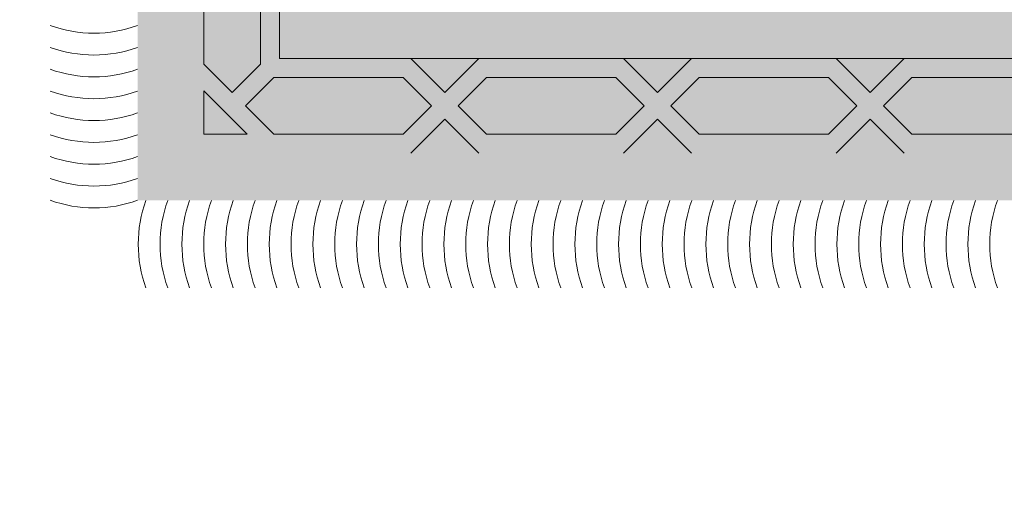
# Model space of a CAD drawing. Units: inches. Extents: x 844 to 2234, y 346 to 1084.
# Tile 8 of 93: x 1114.25 to 1127.54, y 680.17 to 686.54. Entities that reach past the tile are written whole.
import ezdxf

# ---------------------------------------------------------------- set-up
doc = ezdxf.new("R2010")
doc.units = ezdxf.units.IN
doc.header["$MEASUREMENT"] = 0
for name, color, linetype, lineweight in [('A-ANNO-DIMS', 2, 'Continuous', 18), ('furniture', 8, 'Continuous', 18), ('RA-AP-01$0$INT', 35, 'Continuous', 5)]:
    doc.layers.add(name, color=color, linetype=linetype, lineweight=lineweight)
doc.layers.add('RA-AP-01$0$FURN', color=3, linetype='Continuous')
doc.styles.get("Standard").update_dxf_attribs({"font": 'arial.ttf'})
doc.dimstyles.get("Standard").update_dxf_attribs({"dimtxt": 6, "dimasz": 3, "dimexe": 0.18, "dimexo": 0.0625, "dimgap": 0.09, "dimtad": 0, "dimtih": 1, "dimtoh": 1, "dimdec": 1, "dimzin": 0, "dimdsep": 46, "dimlunit": 3, "dimtxsty": 'Standard', "dimblk": 'ARCHTICK', "dimcen": 0.09, "dimadec": 0, "dimazin": 0, "dimtfac": 1, "dimtdec": 1, "dimtofl": 0, "dimtmove": 0, "dimatfit": 3, "dimfxl": 1, "dimtolj": 1, "dimtzin": 0, "dimarcsym": 0})

# ---------------------------------------------------------------- blocks, each defined once
blk = doc.blocks.new('A$C18D01794')
at = {"layer": 'RA-AP-01$0$INT'}
h = blk.add_hatch(color=256, dxfattribs=at)
h.paths.add_polyline_path([(4.3552, -6.1567), (4.3552, -8.0567), (5.4552, -8.0567), (5.4552, -6.1567)])
h.paths.add_polyline_path([(4.4052, -8.0067), (4.4052, -6.2067), (5.4052, -6.2067), (5.4052, -8.0067)], flags=16)
h = blk.add_hatch(color=256, dxfattribs=at)
h.paths.add_polyline_path([(4.4693, -7.0709), (4.5052, -7.035), (4.5052, -7.1067)])
h.paths.add_polyline_path([(4.4552, -7.085), (4.4769, -7.1067), (4.4335, -7.1067)])
h.paths.add_polyline_path([(4.4052, -7.035), (4.4411, -7.0709), (4.4052, -7.1067)])
h.paths.add_polyline_path([(4.4252, -6.9115), (4.4552, -6.8815), (4.4852, -6.9115), (4.4852, -7.0267), (4.4552, -7.0567), (4.4252, -7.0267)])
h.paths.add_polyline_path([(4.5052, -6.8315), (4.5052, -6.9032), (4.4693, -6.8673)])
h.paths.add_polyline_path([(4.4252, -6.7079), (4.4552, -6.6779), (4.4852, -6.7079), (4.4852, -6.8232), (4.4552, -6.8532), (4.4252, -6.8232)])
h.paths.add_polyline_path([(4.4252, -6.5044), (4.4552, -6.4744), (4.4852, -6.5044), (4.4852, -6.6196), (4.4552, -6.6496), (4.4252, -6.6196)])
h.paths.add_polyline_path([(4.4693, -6.6638), (4.5052, -6.6279), (4.5052, -6.6996)])
h.paths.add_polyline_path([(4.4052, -6.6279), (4.4411, -6.6638), (4.4052, -6.6996)])
h.paths.add_polyline_path([(4.4052, -6.4244), (4.4411, -6.4602), (4.4052, -6.4961)])
h.paths.add_polyline_path([(4.4693, -6.4602), (4.5052, -6.4244), (4.5052, -6.4961)])
h.paths.add_polyline_path([(4.4252, -6.3009), (4.4552, -6.2709), (4.4852, -6.3009), (4.4852, -6.4161), (4.4552, -6.4461), (4.4252, -6.4161)])
h.paths.add_polyline_path([(4.4252, -6.2267), (4.4711, -6.2267), (4.4252, -6.2726)])
h.paths.add_polyline_path([(4.4993, -6.2267), (4.6361, -6.2267), (4.6661, -6.2567), (4.6361, -6.2867), (4.4993, -6.2867), (4.4693, -6.2567)])
h.paths.add_polyline_path([(4.6802, -6.2709), (4.7161, -6.3067), (4.6443, -6.3067)])
h.paths.add_polyline_path([(4.6443, -6.2067), (4.7161, -6.2067), (4.6802, -6.2426)])
h.paths.add_polyline_path([(4.7243, -6.2267), (4.8611, -6.2267), (4.8911, -6.2567), (4.8611, -6.2867), (4.7243, -6.2867), (4.6943, -6.2567)])
h.paths.add_polyline_path([(4.9052, -6.2709), (4.9411, -6.3067), (4.8693, -6.3067)])
h.paths.add_polyline_path([(4.8693, -6.2067), (4.9411, -6.2067), (4.9052, -6.2426)])
h.paths.add_polyline_path([(4.9493, -6.2267), (5.0861, -6.2267), (5.1161, -6.2567), (5.0861, -6.2867), (4.9493, -6.2867), (4.9193, -6.2567)])
h.paths.add_polyline_path([(5.1302, -6.2709), (5.1661, -6.3067), (5.0943, -6.3067)])
h.paths.add_polyline_path([(5.0943, -6.2067), (5.1661, -6.2067), (5.1302, -6.2426)])
h.paths.add_polyline_path([(5.1743, -6.2267), (5.3111, -6.2267), (5.3411, -6.2567), (5.3111, -6.2867), (5.1743, -6.2867), (5.1443, -6.2567)])
h.paths.add_polyline_path([(5.3252, -6.3009), (5.3552, -6.2709), (5.3852, -6.3009), (5.3852, -6.4161), (5.3552, -6.4461), (5.3252, -6.4161)])
h.paths.add_polyline_path([(5.3393, -6.2267), (5.3852, -6.2267), (5.3852, -6.2726)])
h.paths.add_polyline_path([(5.3252, -6.5044), (5.3552, -6.4744), (5.3852, -6.5044), (5.3852, -6.6196), (5.3552, -6.6496), (5.3252, -6.6196)])
h.paths.add_polyline_path([(5.3052, -6.4244), (5.3411, -6.4602), (5.3052, -6.4961)])
h.paths.add_polyline_path([(5.3693, -6.4602), (5.4052, -6.4244), (5.4052, -6.4961)])
h.paths.add_polyline_path([(5.4052, -6.6279), (5.4052, -6.6996), (5.3693, -6.6638)])
h.paths.add_polyline_path([(5.3052, -6.6279), (5.3411, -6.6638), (5.3052, -6.6996)])
h.paths.add_polyline_path([(5.3252, -6.7079), (5.3552, -6.6779), (5.3852, -6.7079), (5.3852, -6.8232), (5.3552, -6.8532), (5.3252, -6.8232)])
h.paths.add_polyline_path([(5.3052, -6.8315), (5.3411, -6.8673), (5.3052, -6.9032)])
h.paths.add_polyline_path([(5.3252, -6.9115), (5.3552, -6.8815), (5.3852, -6.9115), (5.3852, -7.0267), (5.3552, -7.0567), (5.3252, -7.0267)])
h.paths.add_polyline_path([(5.4046, -6.8321, 0.001218), (5.4052, -6.8323), (5.4052, -6.9032), (5.3693, -6.8673)])
h.paths.add_polyline_path([(5.3693, -7.0709), (5.4052, -7.035), (5.4052, -7.1067)])
h.paths.add_polyline_path([(5.3552, -7.085), (5.3769, -7.1067), (5.3335, -7.1067)])
h.paths.add_polyline_path([(5.3052, -7.035), (5.3411, -7.0709), (5.3052, -7.1067)])
h = blk.add_hatch(color=256, dxfattribs=at)
h.paths.add_polyline_path([(4.5052, -6.6279), (4.4693, -6.6638), (4.5052, -6.6996), (4.5052, -6.8315), (4.4693, -6.8673), (4.5052, -6.9032), (4.5052, -7.035), (4.4693, -7.0709), (4.5052, -7.1067), (4.4769, -7.1067), (4.4552, -7.085), (4.4335, -7.1067), (4.4052, -7.1067), (4.4411, -7.0709), (4.4052, -7.035), (4.4052, -6.9032), (4.4411, -6.8673), (4.4052, -6.8315), (4.4052, -6.6996), (4.4411, -6.6638), (4.4052, -6.6279), (4.4052, -6.4961), (4.4411, -6.4602), (4.4052, -6.4244), (4.4052, -6.2067), (4.6443, -6.2067), (4.6802, -6.2426), (4.7161, -6.2067), (4.8693, -6.2067), (4.9052, -6.2426), (4.9411, -6.2067), (5.0943, -6.2067), (5.1302, -6.2426), (5.1661, -6.2067), (5.4052, -6.2067), (5.4052, -6.4244), (5.3693, -6.4602), (5.4052, -6.4961), (5.4052, -6.6279), (5.3693, -6.6638), (5.4052, -6.6996), (5.4052, -6.8315), (5.3693, -6.8673), (5.4052, -6.9032), (5.4052, -7.035), (5.3693, -7.0709), (5.4052, -7.1067), (5.3769, -7.1067), (5.3552, -7.085), (5.3335, -7.1067), (5.3052, -7.1067), (5.3411, -7.0709), (5.3052, -7.035), (5.3052, -6.9032), (5.3411, -6.8673), (5.3052, -6.8315), (5.3052, -6.6996), (5.3411, -6.6638), (5.3052, -6.6279), (5.3052, -6.4961), (5.3411, -6.4602), (5.3052, -6.4244), (5.3052, -6.3067), (5.1661, -6.3067), (5.1302, -6.2709), (5.0943, -6.3067), (4.9411, -6.3067), (4.9052, -6.2709), (4.8693, -6.3067), (4.7161, -6.3067), (4.6802, -6.2709), (4.6443, -6.3067), (4.5052, -6.3067), (4.5052, -6.4244), (4.4693, -6.4602), (4.5052, -6.4961)])
h.paths.add_polyline_path([(4.4852, -6.5044), (4.4552, -6.4744), (4.4252, -6.5044), (4.4252, -6.6196), (4.4552, -6.6496), (4.4852, -6.6196)], flags=16)
h.paths.add_polyline_path([(4.4552, -6.4461), (4.4852, -6.4161), (4.4852, -6.3009), (4.4552, -6.2709), (4.4252, -6.3009), (4.4252, -6.4161)], flags=16)
h.paths.add_polyline_path([(4.4552, -6.6779), (4.4252, -6.7079), (4.4252, -6.8232), (4.4552, -6.8532), (4.4852, -6.8232), (4.4852, -6.7079)], flags=16)
h.paths.add_polyline_path([(4.4993, -6.2867), (4.6361, -6.2867), (4.6661, -6.2567), (4.6361, -6.2267), (4.4993, -6.2267), (4.4693, -6.2567)], flags=16)
h.paths.add_polyline_path([(4.4252, -6.2726), (4.4711, -6.2267), (4.4252, -6.2267)], flags=16)
h.paths.add_polyline_path([(4.4552, -6.8815), (4.4252, -6.9115), (4.4252, -7.0267), (4.4552, -7.0567), (4.4852, -7.0267), (4.4852, -6.9115)], flags=16)
h.paths.add_polyline_path([(4.7243, -6.2867), (4.8611, -6.2867), (4.8911, -6.2567), (4.8611, -6.2267), (4.7243, -6.2267), (4.6943, -6.2567)], flags=16)
h.paths.add_polyline_path([(4.9193, -6.2567), (4.9493, -6.2867), (5.0861, -6.2867), (5.1161, -6.2567), (5.0861, -6.2267), (4.9493, -6.2267)], flags=16)
h.paths.add_polyline_path([(5.1443, -6.2567), (5.1743, -6.2867), (5.3111, -6.2867), (5.3411, -6.2567), (5.3111, -6.2267), (5.1743, -6.2267)], flags=16)
h.paths.add_polyline_path([(5.3252, -6.6196), (5.3552, -6.6496), (5.3852, -6.6196), (5.3852, -6.5044), (5.3552, -6.4744), (5.3252, -6.5044)], flags=16)
h.paths.add_polyline_path([(5.3252, -6.4161), (5.3552, -6.4461), (5.3852, -6.4161), (5.3852, -6.3009), (5.3552, -6.2709), (5.3252, -6.3009)], flags=16)
h.paths.add_polyline_path([(5.3252, -6.7079), (5.3252, -6.8232), (5.3552, -6.8532), (5.3852, -6.8232), (5.3852, -6.7079), (5.3552, -6.6779)], flags=16)
h.paths.add_polyline_path([(5.3252, -6.9115), (5.3252, -7.0267), (5.3552, -7.0567), (5.3852, -7.0267), (5.3852, -6.9115), (5.3552, -6.8815)], flags=16)
h.paths.add_polyline_path([(5.3393, -6.2267), (5.3852, -6.2726), (5.3852, -6.2267)], flags=16)
blk.add_hatch(color=256, dxfattribs=at).paths.add_polyline_path([(4.5052, -6.3067), (5.3052, -6.3067), (5.3052, -7.1067), (5.2552, -7.1067), (5.2552, -6.3567), (4.5552, -6.3567), (4.5552, -7.1067), (4.5052, -7.1067)])
for p, q in [((4.6443, -6.2067), (4.6802, -6.2426)), ((4.7161, -6.2067), (4.6802, -6.2426)), ((4.8693, -6.2067), (4.9052, -6.2426)), ((4.9411, -6.2067), (4.9052, -6.2426)), ((5.0943, -6.2067), (5.1302, -6.2426)), ((5.1661, -6.2067), (5.1302, -6.2426)), ((4.4711, -6.2267), (4.4252, -6.2726)), ((4.4252, -6.2726), (4.4252, -6.2267)), ((4.4711, -6.2267), (4.4252, -6.2267)), ((4.4993, -6.2267), (4.4693, -6.2567)), ((4.6361, -6.2267), (4.4993, -6.2267)), ((4.6361, -6.2267), (4.6661, -6.2567)), ((4.7243, -6.2267), (4.6943, -6.2567)), ((4.8611, -6.2267), (4.7243, -6.2267)), ((4.8611, -6.2267), (4.8911, -6.2567)), ((4.9493, -6.2267), (4.9193, -6.2567)), ((4.9493, -6.2267), (5.0861, -6.2267)), ((5.0861, -6.2267), (5.1161, -6.2567)), ((5.1743, -6.2267), (5.1443, -6.2567)), ((5.1743, -6.2267), (5.3111, -6.2267)), ((4.4993, -6.2867), (4.4693, -6.2567)), ((4.6361, -6.2867), (4.6661, -6.2567)), ((4.7243, -6.2867), (4.6943, -6.2567)), ((4.8611, -6.2867), (4.8911, -6.2567)), ((4.9493, -6.2867), (4.9193, -6.2567)), ((5.0861, -6.2867), (5.1161, -6.2567)), ((5.1743, -6.2867), (5.1443, -6.2567)), ((4.4252, -6.3009), (4.4552, -6.2709)), ((4.4852, -6.3009), (4.4552, -6.2709)), ((4.6443, -6.3067), (4.6802, -6.2709)), ((4.7161, -6.3067), (4.6802, -6.2709)), ((4.8693, -6.3067), (4.9052, -6.2709)), ((4.9411, -6.3067), (4.9052, -6.2709)), ((5.0943, -6.3067), (5.1302, -6.2709)), ((5.1661, -6.3067), (5.1302, -6.2709)), ((4.6361, -6.2867), (4.4993, -6.2867)), ((4.8611, -6.2867), (4.7243, -6.2867)), ((4.9493, -6.2867), (5.0861, -6.2867)), ((5.1743, -6.2867), (5.3111, -6.2867)), ((4.4252, -6.4161), (4.4252, -6.3009)), ((4.4852, -6.3009), (4.4852, -6.4161)), ((5.2672, -6.3067), (4.5432, -6.3067)), ((5.2672, -6.3067), (4.5432, -6.3067))]:
    blk.add_line(p, q, dxfattribs=at)
blk.add_lwpolyline([(5.3052, -7.1067), (5.3052, -6.3067), (4.5052, -6.3067), (4.5052, -7.1067)], dxfattribs=at)
for centre, start, end in [((4.4922, -6.1105), 160.2038, 199.7962), ((4.5153, -6.1105), 160.2038, 199.7962), ((4.5384, -6.1105), 160.2038, 199.7962), ((4.5615, -6.1105), 160.2038, 199.7962), ((4.5846, -6.1105), 160.2038, 199.7962), ((4.6077, -6.1105), 160.2038, 199.7962), ((4.6308, -6.1105), 160.2038, 199.7962), ((4.6539, -6.1105), 160.2038, 199.7962), ((4.677, -6.1105), 160.2038, 199.7962), ((4.7001, -6.1105), 160.2038, 199.7962), ((4.7232, -6.1105), 160.2038, 199.7962), ((4.7463, -6.1105), 160.2038, 199.7962), ((4.7694, -6.1105), 160.2038, 199.7962), ((4.7925, -6.1105), 160.2038, 199.7962), ((4.8156, -6.1105), 160.2038, 199.7962), ((4.8387, -6.1105), 160.2038, 199.7962), ((4.8618, -6.1105), 160.2038, 199.7962), ((4.8849, -6.1105), 160.2038, 199.7962), ((4.908, -6.1105), 160.2038, 199.7962), ((4.9311, -6.1105), 160.2038, 199.7962), ((4.9542, -6.1105), 160.2038, 199.7962), ((4.9773, -6.1105), 160.2038, 199.7962), ((5.0004, -6.1105), 160.2038, 199.7962), ((5.0235, -6.1105), 160.2038, 199.7962), ((5.0466, -6.1105), 160.2038, 199.7962), ((5.0697, -6.1105), 160.2038, 199.7962), ((5.0928, -6.1105), 160.2038, 199.7962), ((5.1159, -6.1105), 160.2038, 199.7962), ((5.139, -6.1105), 160.2038, 199.7962), ((5.1621, -6.1105), 160.2038, 199.7962), ((5.1852, -6.1105), 160.2038, 199.7962), ((5.2083, -6.1105), 160.2038, 199.7962), ((5.2314, -6.1105), 160.2038, 199.7962), ((5.2545, -6.1105), 160.2038, 199.7962), ((5.2776, -6.1105), 160.2038, 199.7962), ((5.3007, -6.1105), 160.2038, 199.7962), ((5.3238, -6.1105), 160.2038, 199.7962), ((5.3469, -6.1105), 160.2038, 199.7962), ((5.37, -6.1105), 160.2038, 199.7962), ((5.3931, -6.1105), 160.2038, 199.7962), ((4.309, -6.2852), 70.2038, 109.7962), ((4.309, -6.3083), 70.2038, 109.7962), ((4.309, -6.3314), 70.2038, 109.7962), ((4.309, -6.3545), 70.2038, 109.7962), ((4.309, -6.3776), 70.2038, 109.7962), ((4.309, -6.4007), 70.2038, 109.7962), ((4.309, -6.4238), 70.2038, 109.7962), ((4.309, -6.4469), 70.2038, 109.7962), ((4.309, -6.47), 70.2038, 109.7962)]:
    blk.add_arc(centre, 0.1364, start, end, dxfattribs=at)
blk = doc.blocks.new('A$C5D2F253E')
at = {"layer": 'RA-AP-01$0$FURN', "xscale": -0.7999999999883585, "yscale": 0.7999999999883585, "zscale": 0.8, "rotation": 90}
blk.add_blockref('A$C18D01794', (-5.68776, 4.75792), dxfattribs=at)
blk = doc.blocks.new('_ArchTick')
at = {"color": 0, "linetype": 'ByBlock', "const_width": 0.15}
blk.add_lwpolyline([(-0.5, -0.5), (0.5, 0.5)], dxfattribs=at)
blk = doc.blocks.new('*D144')
at = {"layer": 'A-ANNO-DIMS', "color": 0, "lineweight": -2, "transparency": 16777216}
for p, q in [((1096.616, 439.373), (1096.616, 1074.743)), ((1143.116, 492.373), (1143.116, 1074.743)), ((1096.616, 1074.563), (1102.482, 1074.563)), ((1143.116, 1074.563), (1137.25, 1074.563))]:
    blk.add_line(p, q, dxfattribs=at)
at = {"layer": 'Defpoints', "color": 0, "transparency": 16777216}
for p in [(1143.116, 1074.563), (1143.116, 492.311), (1096.616, 439.311)]:
    blk.add_point(p, dxfattribs=at)
at = {"layer": 'A-ANNO-DIMS', "color": 0, "lineweight": -2, "transparency": 16777216, "xscale": 3, "yscale": 3, "zscale": 3, "rotation": 180}
blk.add_blockref('_ArchTick', (1096.616, 1074.563), dxfattribs=at)
at = {"layer": 'A-ANNO-DIMS', "color": 0, "lineweight": -2, "transparency": 16777216, "xscale": 3, "yscale": 3, "zscale": 3}
blk.add_blockref('_ArchTick', (1143.116, 1074.563), dxfattribs=at)
at = {"layer": 'A-ANNO-DIMS', "color": 0, "transparency": 16777216, "insert": (1119.866, 1074.563), "char_height": 6, "attachment_point": 5}
blk.add_mtext('\\A1;3\'-10 1/2"', dxfattribs=at)

msp = doc.modelspace()

# ---------------------------------------------------------------- block references
at = {"layer": 'furniture', "xscale": 15.94108302203742, "yscale": 15.94108302203742, "zscale": 15.94108302203742, "rotation": 90}
msp.add_blockref('A$C5D2F253E', (1136.148, 696.258), dxfattribs=at)

# ---------------------------------------------------------------- dimensions: what is measured, and where the dimension line sits
at = {"layer": 'A-ANNO-DIMS'}
dim = msp.add_linear_dim(base=(1143.116, 1074.563), p1=(1096.616, 439.311), p2=(1143.116, 492.311), dimstyle='Standard', override={"dimdec": 1, "dimlfac": 1, "dimrnd": 0, "dimzin": 1, "dimdsep": 46, "dimlunit": 4, "dimfrac": 2}, dxfattribs=at)
dim.commit()
dim.dimension.update_dxf_attribs({"geometry": '*D144', "text_midpoint": (1119.866, 1074.563)})

doc.saveas('drawing.dxf')
